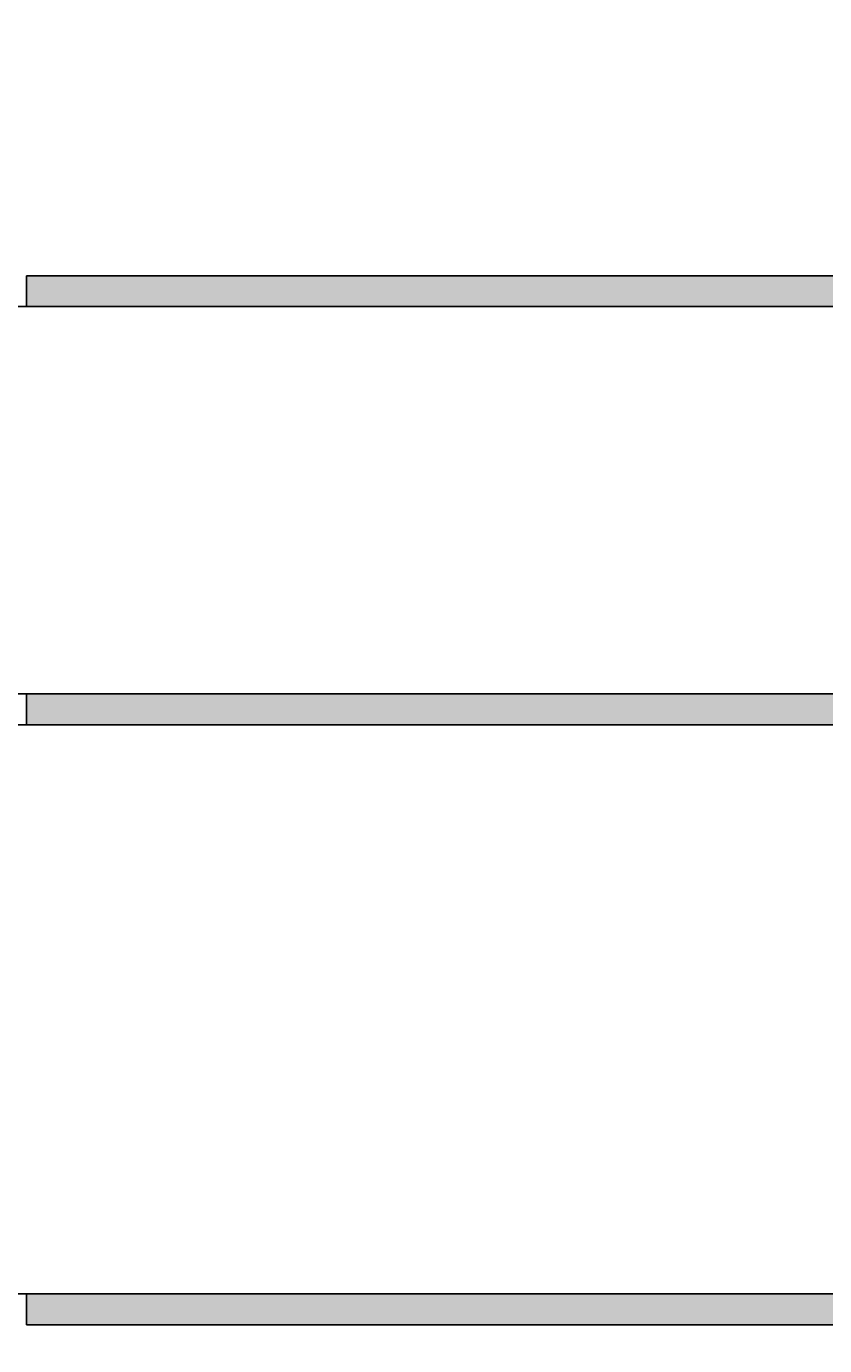
# Model space of a CAD drawing. Units: inches. Extents: x 35362 to 73946, y 43607 to 67532.
# Tile 133 of 134: x 68484 to 69000, y 45436 to 46290. Entities that reach past the tile are written whole.
import ezdxf

# ---------------------------------------------------------------- set-up
doc = ezdxf.new("R2010")
doc.units = ezdxf.units.IN
doc.header["$MEASUREMENT"] = 0
for name, color, linetype, lineweight in [('A-ANNO-DIMS', 2, 'Continuous', 18), ('E-SYMB', 1, 'Continuous', 25), ('E-SYMB-PATT', 1, 'Continuous', 13)]:
    doc.layers.add(name, color=color, linetype=linetype, lineweight=lineweight)
doc.styles.get("Standard").update_dxf_attribs({"font": 'arial.ttf'})
doc.dimstyles.get("Standard").update_dxf_attribs({"dimtxt": 0.18, "dimasz": 0.18, "dimexe": 0.18, "dimexo": 0.0625, "dimgap": 0.09, "dimtad": 0, "dimtih": 1, "dimtoh": 1, "dimdec": 4, "dimzin": 0, "dimdsep": 46, "dimtxsty": 'Standard', "dimcen": 0.09, "dimadec": 0, "dimazin": 0, "dimtfac": 1, "dimtdec": 4, "dimtofl": 0, "dimtmove": 0, "dimatfit": 3, "dimfxl": 1, "dimtolj": 1, "dimtzin": 0, "dimarcsym": 0})

# ---------------------------------------------------------------- blocks, each defined once
blk = doc.blocks.new('CT-CORE')
for p, q in [((-0.0004610742907971, 1387.996120092102), (-0.0004610742907971, -5.34733626409e-05)), ((19.9995389257092, -5.34733626409e-05), (19.99953892572375, 1387.996120092102)), ((270.6681283192447, 1387.996120092102), (270.6681283192447, -5.34733626409e-05)), ((290.6681283192447, -5.34733626409e-05), (290.6681283192593, 1387.996120092102)), ((658.9826659540267, 544.3844491987692), (658.9826659540267, -5.34733626409e-05)), ((678.9826659540267, -5.34733626409e-05), (678.9826659540413, 543.5352826863744)), ((-0.0004610742907971, -5.34733626409e-05), (19.9995389257092, -5.34733626409e-05)), ((270.6681283192447, -5.34733626409e-05), (290.6681283192447, -5.34733626409e-05)), ((658.9826659540267, -5.34733626409e-05), (678.9826659540267, -5.34733626409e-05))]:
    blk.add_line(p, q)
blk = doc.blocks.new('*D5')
at = {"layer": 'A-ANNO-DIMS', "color": 0, "lineweight": -2, "transparency": 16777216}
for p, q in [((37121.949085, 46919.318283), (37121.949085, 43606.678996)), ((69871.496302, 45449.831951), (69871.496302, 43606.678996)), ((37122.129085, 43606.858996), (53496.2943647142, 43606.858996)), ((69871.316302, 43606.858996), (53497.15102228581, 43606.858996))]:
    blk.add_line(p, q, dxfattribs=at)
at = {"layer": 'A-ANNO-DIMS', "color": 0, "transparency": 16777216}
for points in [[(37122.129085, 43606.888996), (37122.129085, 43606.828996), (37121.949085, 43606.858996)], [(69871.316302, 43606.888996), (69871.316302, 43606.828996), (69871.496302, 43606.858996)]]:
    blk.add_solid(points, dxfattribs=at)
at = {"layer": 'Defpoints', "color": 0, "transparency": 16777216}
for p in [(37121.949085, 46919.380783), (69871.496302, 45449.894451), (69871.496302, 43606.858996)]:
    blk.add_point(p, dxfattribs=at)
at = {"layer": 'A-ANNO-DIMS', "color": 0, "transparency": 16777216, "insert": (53496.7226935, 43606.858996), "char_height": 0.18, "attachment_point": 5}
blk.add_mtext('\\A1;32750', dxfattribs=at)
blk = doc.blocks.new('*D74')
at = {"layer": 'A-ANNO-DIMS', "color": 0, "lineweight": -2, "transparency": 16777216}
for p, q in [((55181.69646300003, 46108.87757800001), (73945.82566600003, 46108.87757800001)), ((73945.64566600005, 46108.69757800001), (73945.64566600005, 45983.7251866378)), ((73945.64566600005, 45858.38898900001), (73945.64566600005, 45983.36138036223)), ((55181.69646300003, 45858.20898900001), (73945.82566600003, 45858.20898900001))]:
    blk.add_line(p, q, dxfattribs=at)
at = {"layer": 'A-ANNO-DIMS', "color": 0, "transparency": 16777216}
for points in [[(73945.61566600006, 46108.69757800001), (73945.67566600005, 46108.69757800001), (73945.64566600005, 46108.87757800001)], [(73945.61566600006, 45858.38898900001), (73945.67566600005, 45858.38898900001), (73945.64566600005, 45858.20898900001)]]:
    blk.add_solid(points, dxfattribs=at)
at = {"layer": 'Defpoints', "color": 0, "transparency": 16777216}
for p in [(55181.63396300002, 46108.87757800001), (55181.63396300002, 45858.20898900001), (73945.64566600005, 45858.20898900001)]:
    blk.add_point(p, dxfattribs=at)
at = {"layer": 'A-ANNO-DIMS', "color": 0, "transparency": 16777216, "insert": (73945.64566600005, 45983.54328349999), "char_height": 0.18, "attachment_point": 5}
blk.add_mtext('\\A1;250.67', dxfattribs=at)
blk = doc.blocks.new('*D75')
at = {"layer": 'A-ANNO-DIMS', "color": 0, "lineweight": -2, "transparency": 16777216}
for p, q in [((55181.69646300003, 45838.20898900001), (73945.82566600003, 45838.20898900001)), ((73945.64566600005, 45838.02898900001), (73945.64566600005, 45654.23368452933)), ((73945.64566600005, 45470.07445100001), (73945.64566600005, 45653.86975547068)), ((55181.69646300003, 45469.89445100001), (73945.82566600003, 45469.89445100001))]:
    blk.add_line(p, q, dxfattribs=at)
at = {"layer": 'A-ANNO-DIMS', "color": 0, "transparency": 16777216}
for points in [[(73945.61566600006, 45838.02898900001), (73945.67566600005, 45838.02898900001), (73945.64566600005, 45838.20898900001)], [(73945.61566600006, 45470.07445100001), (73945.67566600005, 45470.07445100001), (73945.64566600005, 45469.89445100001)]]:
    blk.add_solid(points, dxfattribs=at)
at = {"layer": 'Defpoints', "color": 0, "transparency": 16777216}
for p in [(55181.63396300002, 45838.20898900001), (55181.63396300002, 45469.89445100001), (73945.64566600005, 45469.89445100001)]:
    blk.add_point(p, dxfattribs=at)
at = {"layer": 'A-ANNO-DIMS', "color": 0, "transparency": 16777216, "insert": (73945.64566600005, 45654.05171999998), "char_height": 0.18, "attachment_point": 5}
blk.add_mtext('\\A1;368.3', dxfattribs=at)

msp = doc.modelspace()

# ---------------------------------------------------------------- hatches: boundary and pattern name
at = {"layer": 'E-SYMB-PATT'}
h = msp.add_hatch(color=256, dxfattribs=at)
h.dxf.hatch_style = 1
h.paths.add_polyline_path([(69871.49630189747, 46108.87757831767), (69871.49630189747, 46128.87757831768), (68483.50012833202, 46128.87757831768), (68483.50012833202, 46108.87757831768)])
h = msp.add_hatch(color=256, dxfattribs=at)
h.dxf.hatch_style = 1
h.paths.add_polyline_path([(69871.49630189747, 45838.20898892413), (69871.49630189747, 45858.20898892414), (68483.50012833202, 45858.20898892414), (68483.50012833202, 45838.20898892414)])
h = msp.add_hatch(color=256, dxfattribs=at)
h.dxf.hatch_style = 1
h.paths.add_polyline_path([(69027.03546449174, 45449.89445128935, -0.0212196039209565), (69027.88463100414, 45469.89445128936), (69011.01171653513, 45469.89445128936, 0.0200709024740955), (69010.20855689044, 45449.89445128935)])
h.paths.add_polyline_path([(69010.20855689044, 45449.89445128935, -0.0200709024740953), (69011.01171653513, 45469.89445128936), (68483.50012833202, 45469.89445128936), (68483.50012833202, 45449.89445128936)])
h.paths.add_polyline_path([(69871.49630189747, 45449.89445128935), (69871.49630189747, 45469.89445128936), (69508.24154776601, 45469.89445128936, -0.0200709024740959), (69509.04470741072, 45449.89445128935)])
h.paths.add_polyline_path([(69509.04470741072, 45449.89445128935, 0.020070902474096), (69508.24154776601, 45469.89445128936), (69498.08559913776, 45469.89445128936, -0.0212196039209564), (69498.93476565015, 45449.89445128935)])

# ---------------------------------------------------------------- block references
at = {"layer": 'E-SYMB', "rotation": 269.9999999999974}
msp.add_blockref('CT-CORE', (68483.50018180539, 46128.87711724339), dxfattribs=at)

# ---------------------------------------------------------------- dimensions: what is measured, and where the dimension line sits
at = {"layer": 'A-ANNO-DIMS'}
dim = msp.add_linear_dim(base=(69871.496302, 43606.858996), p1=(37121.949085, 46919.380783), p2=(69871.496302, 45449.894451), dimstyle='Standard', override={"dimdec": 0, "dimlfac": 1, "dimrnd": 0, "dimzin": 0, "dimdsep": 46, "dimlunit": 2}, dxfattribs=at)
dim.commit()
dim.dimension.update_dxf_attribs({"geometry": '*D5', "text_midpoint": (53496.7226935, 43606.858996)})
for base, p1, p2, override, picture, middle in [((73945.64566600005, 45858.20898900001), (55181.633963, 46108.877578), (55181.633963, 45858.20898899999), {"dimdec": 2, "dimlfac": 1, "dimrnd": 0, "dimzin": 0, "dimdsep": 46, "dimlunit": 2}, '*D74', (73945.64566600005, 45983.54328349999)), ((73945.64566600005, 45469.89445100001), (55181.633963, 45838.20898899999), (55181.633963, 45469.894451), {"dimdec": 1, "dimlfac": 1, "dimrnd": 0, "dimzin": 0, "dimdsep": 46, "dimlunit": 2}, '*D75', (73945.64566600005, 45654.05171999998))]:
    dim = msp.add_linear_dim(base=base, p1=p1, p2=p2, angle=90, dimstyle='Standard', override=override, dxfattribs=at)
    dim.commit()
    dim.dimension.update_dxf_attribs({"geometry": picture, "text_midpoint": middle})

doc.saveas('drawing.dxf')
